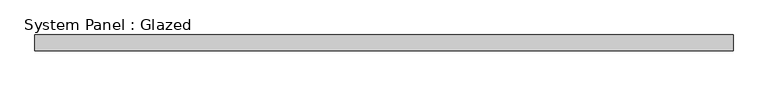
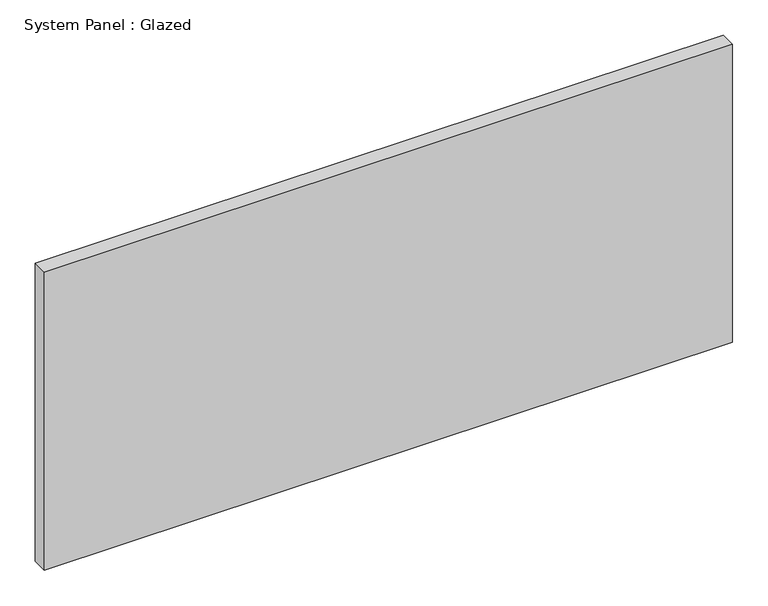
"""IFC4 building model written with IfcOpenShell, lengths in millimetres: plate geometry, System Panel : Glazed."""

from ifc_helpers import new_model, si_unit, origin, origin_with_axes, place, context, project, spatial, polyline, outline, extrude, source, transform, mapped, element, save


def system_panel_glazed_738ee2ab(model_context):
    return source(origin(), model_context, "Body", "SweptSolid", [
        extrude(outline(polyline([(561.975, -44.45), (-561.975, -44.45), (-561.975, -19.05), (561.975, -19.05), (561.975, -44.45)])), origin_with_axes(), (0.0, 0.0, 1.0), 514.35),
    ])


if __name__ == "__main__":
    model = new_model("IFC4")
    model_context = context("Model", 3, world=origin())
    ifc_project = project(units=[si_unit("LENGTHUNIT", "METRE", prefix="MILLI")], contexts=[model_context])
    site = spatial("IfcSite", under=ifc_project)
    building = spatial("IfcBuilding", under=site)
    placement = place(None, origin())
    system_panel_glazed_shape = system_panel_glazed_738ee2ab(model_context)
    element("IfcPlate", 1, ObjectType="System Panel : Glazed", at=placement, inside=building, context=model_context, shape_type="MappedRepresentation", body=[
        mapped(system_panel_glazed_shape, transform((0.0, 0.0, 0.0), x_axis=(1.0, 0.0, 0.0), y_axis=(0.0, 1.0, 0.0), z_axis=(0.0, 0.0, 1.0))),
    ])
    save(model, "model.ifc")

# Revit data of these elements
# Type "System Panel : Glazed"
#   Construction Type Id = "GSP4R"
#   Analytic Construction = "1/8 in Pilkington single glazing"
#   Visual Light Transmittance = 0.9
#   Solar Heat Gain Coefficient = 0.86
#   Heat Transfer Coefficient (U) = 1.18115 BTU/(h·ft²·°F)
#   Define Thermal Properties by = 1
# Element 1 (IfcPlate, "System Panel : Glazed")
#   Materials on its faces: "GARAGE PANEL"
# Materials
#   "GARAGE PANEL": class "Generic", colour RGB 120 120 120, transparency 0, Cost = 0
